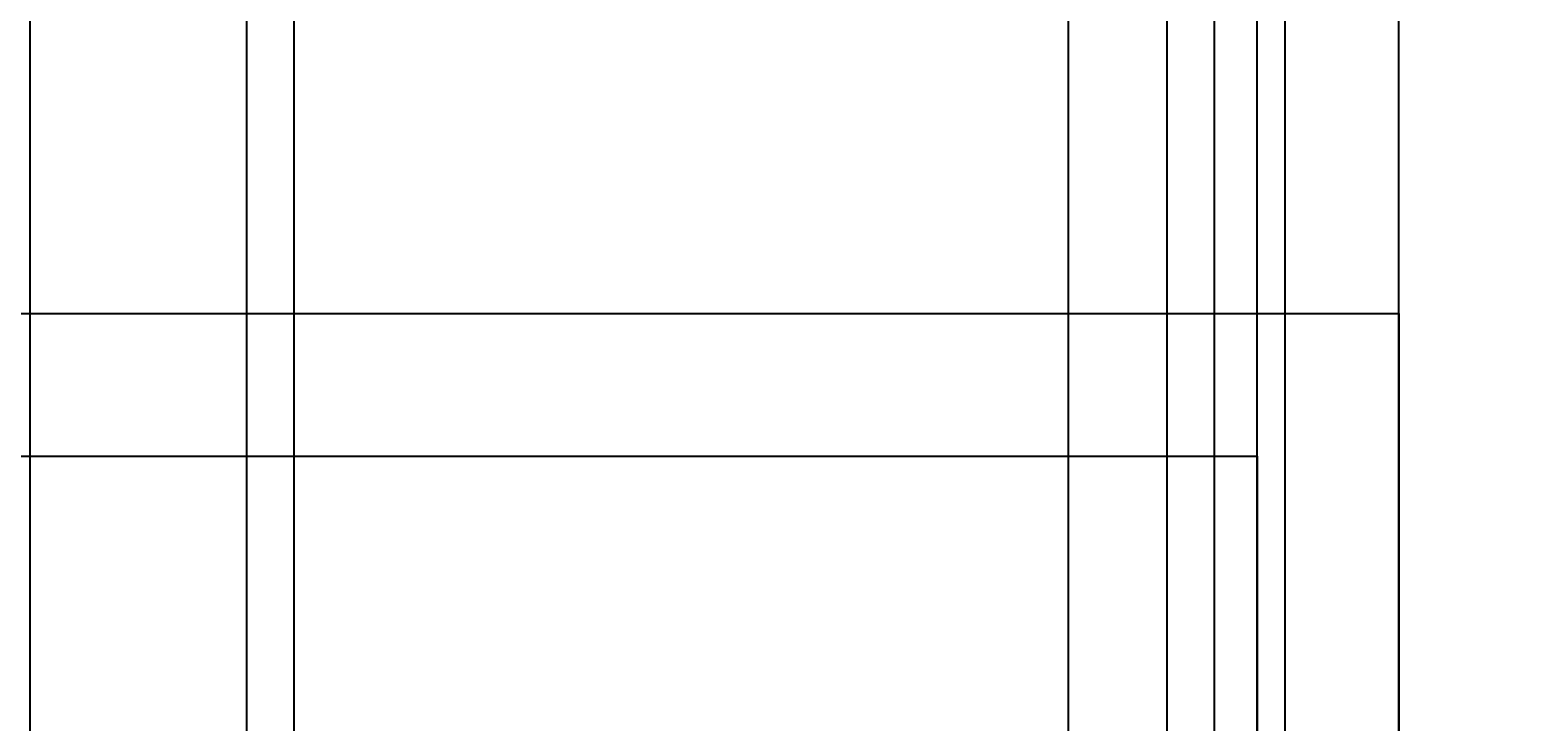
# Model space of a CAD drawing. Units: inches. Extents: x -6 to 289, y -8 to 323.
# Tile 27 of 107: x 142 to 174, y 109 to 124. Entities that reach past the tile are written whole.
import ezdxf

# ---------------------------------------------------------------- set-up
doc = ezdxf.new("R2010")
doc.units = ezdxf.units.IN
doc.header["$MEASUREMENT"] = 0
doc.layers.add('A-ANNO-DIMS', color=2, linetype='Continuous', lineweight=18)
doc.layers.add('A-DOOR', color=3, linetype='Continuous', lineweight=25)
doc.styles.get("Standard").update_dxf_attribs({"font": 'arial.ttf'})
doc.dimstyles.get("Standard").update_dxf_attribs({"dimtxt": 0.18, "dimasz": 0.18, "dimexe": 0.18, "dimexo": 0.0625, "dimgap": 0.09, "dimtad": 0, "dimtih": 1, "dimtoh": 1, "dimdec": 4, "dimzin": 0, "dimdsep": 46, "dimtxsty": 'Standard', "dimcen": 0.09, "dimadec": 0, "dimazin": 0, "dimtfac": 1, "dimtdec": 4, "dimtofl": 0, "dimtmove": 0, "dimatfit": 3, "dimfxl": 1, "dimtolj": 1, "dimtzin": 0, "dimarcsym": 0})

# ---------------------------------------------------------------- blocks, each defined once
blk = doc.blocks.new('*D30')
at = {"layer": 'A-ANNO-DIMS', "color": 0, "lineweight": -2, "transparency": 16777216}
for p, q in [((129.383, 181.092), (129.383, -8.391)), ((146.883, 181.092), (146.883, -8.391)), ((129.563, -8.211), (137.817, -8.211)), ((146.703, -8.211), (138.449, -8.211))]:
    blk.add_line(p, q, dxfattribs=at)
at = {"layer": 'A-ANNO-DIMS', "color": 0, "transparency": 16777216}
for points in [[(129.563, -8.181), (129.563, -8.241), (129.383, -8.211)], [(146.703, -8.181), (146.703, -8.241), (146.883, -8.211)]]:
    blk.add_solid(points, dxfattribs=at)
at = {"layer": 'Defpoints', "color": 0, "transparency": 16777216}
for p in [(129.383, 181.154), (146.883, 181.154), (146.883, -8.211)]:
    blk.add_point(p, dxfattribs=at)
at = {"layer": 'A-ANNO-DIMS', "color": 0, "transparency": 16777216, "insert": (138.133, -8.211), "char_height": 0.18, "attachment_point": 5}
blk.add_mtext('\\A1;17.5', dxfattribs=at)
blk = doc.blocks.new('*D31')
at = {"layer": 'A-ANNO-DIMS', "color": 0, "lineweight": -2, "transparency": 16777216}
for p, q in [((146.883, 181.092), (146.883, -8.391)), ((147.883, 181.092), (147.883, -8.391)), ((147.063, -8.211), (147.26, -8.211)), ((147.703, -8.211), (147.507, -8.211))]:
    blk.add_line(p, q, dxfattribs=at)
at = {"layer": 'A-ANNO-DIMS', "color": 0, "transparency": 16777216}
for points in [[(147.063, -8.181), (147.063, -8.241), (146.883, -8.211)], [(147.703, -8.181), (147.703, -8.241), (147.883, -8.211)]]:
    blk.add_solid(points, dxfattribs=at)
at = {"layer": 'Defpoints', "color": 0, "transparency": 16777216}
for p in [(146.883, 181.154), (147.883, 181.154), (147.883, -8.211)]:
    blk.add_point(p, dxfattribs=at)
at = {"layer": 'A-ANNO-DIMS', "color": 0, "transparency": 16777216, "insert": (147.383, -8.211), "char_height": 0.18, "attachment_point": 5}
blk.add_mtext('\\A1;1', dxfattribs=at)
blk = doc.blocks.new('*D32')
at = {"layer": 'A-ANNO-DIMS', "color": 0, "lineweight": -2, "transparency": 16777216}
for p, q in [((147.883, 181.092), (147.883, -8.391)), ((166.383, 181.092), (166.383, -8.391)), ((148.063, -8.211), (156.817, -8.211)), ((166.203, -8.211), (157.449, -8.211))]:
    blk.add_line(p, q, dxfattribs=at)
at = {"layer": 'A-ANNO-DIMS', "color": 0, "transparency": 16777216}
for points in [[(148.063, -8.181), (148.063, -8.241), (147.883, -8.211)], [(166.203, -8.181), (166.203, -8.241), (166.383, -8.211)]]:
    blk.add_solid(points, dxfattribs=at)
at = {"layer": 'Defpoints', "color": 0, "transparency": 16777216}
for p in [(147.883, 181.154), (166.383, 181.154), (166.383, -8.211)]:
    blk.add_point(p, dxfattribs=at)
at = {"layer": 'A-ANNO-DIMS', "color": 0, "transparency": 16777216, "insert": (157.133, -8.211), "char_height": 0.18, "attachment_point": 5}
blk.add_mtext('\\A1;18.5', dxfattribs=at)
blk = doc.blocks.new('*D33')
at = {"layer": 'A-ANNO-DIMS', "color": 0, "lineweight": -2, "transparency": 16777216}
for p, q in [((166.383, 181.092), (166.383, -8.391)), ((167.383, 180.092), (167.383, -8.391)), ((166.563, -8.211), (166.76, -8.211)), ((167.203, -8.211), (167.007, -8.211))]:
    blk.add_line(p, q, dxfattribs=at)
at = {"layer": 'A-ANNO-DIMS', "color": 0, "transparency": 16777216}
for points in [[(166.563, -8.181), (166.563, -8.241), (166.383, -8.211)], [(167.203, -8.181), (167.203, -8.241), (167.383, -8.211)]]:
    blk.add_solid(points, dxfattribs=at)
at = {"layer": 'Defpoints', "color": 0, "transparency": 16777216}
for p in [(166.383, 181.154), (167.383, 180.154), (167.383, -8.211)]:
    blk.add_point(p, dxfattribs=at)
at = {"layer": 'A-ANNO-DIMS', "color": 0, "transparency": 16777216, "insert": (166.883, -8.211), "char_height": 0.18, "attachment_point": 5}
blk.add_mtext('\\A1;1', dxfattribs=at)
blk = doc.blocks.new('*D34')
at = {"layer": 'A-ANNO-DIMS', "color": 0, "lineweight": -2, "transparency": 16777216}
for p, q in [((167.383, 180.092), (167.383, -8.391)), ((168.883, 178.592), (168.883, -8.391)), ((167.563, -8.211), (167.887, -8.211)), ((168.703, -8.211), (168.38, -8.211))]:
    blk.add_line(p, q, dxfattribs=at)
at = {"layer": 'A-ANNO-DIMS', "color": 0, "transparency": 16777216}
for points in [[(167.563, -8.181), (167.563, -8.241), (167.383, -8.211)], [(168.703, -8.181), (168.703, -8.241), (168.883, -8.211)]]:
    blk.add_solid(points, dxfattribs=at)
at = {"layer": 'Defpoints', "color": 0, "transparency": 16777216}
for p in [(167.383, 180.154), (168.883, 178.654), (168.883, -8.211)]:
    blk.add_point(p, dxfattribs=at)
at = {"layer": 'A-ANNO-DIMS', "color": 0, "transparency": 16777216, "insert": (168.133, -8.211), "char_height": 0.18, "attachment_point": 5}
blk.add_mtext('\\A1;1.5', dxfattribs=at)
blk = doc.blocks.new('*D76')
at = {"layer": 'A-ANNO-DIMS', "color": 0, "lineweight": -2, "transparency": 16777216}
for p, q in [((142.296, 51.148), (142.296, 322.969)), ((142.476, 322.789), (153.076, 322.789)), ((164.116, 322.789), (153.516, 322.789)), ((164.296, 51.148), (164.296, 322.969))]:
    blk.add_line(p, q, dxfattribs=at)
at = {"layer": 'A-ANNO-DIMS', "color": 0, "transparency": 16777216}
for points in [[(142.476, 322.819), (142.476, 322.759), (142.296, 322.789)], [(164.116, 322.819), (164.116, 322.759), (164.296, 322.789)]]:
    blk.add_solid(points, dxfattribs=at)
at = {"layer": 'Defpoints', "color": 0, "transparency": 16777216}
for p in [(164.296, 322.789), (142.296, 51.085), (164.296, 51.085)]:
    blk.add_point(p, dxfattribs=at)
at = {"layer": 'A-ANNO-DIMS', "color": 0, "transparency": 16777216, "insert": (153.296, 322.789), "char_height": 0.18, "attachment_point": 5}
blk.add_mtext('\\A1;22', dxfattribs=at)
blk = doc.blocks.new('*D77')
at = {"layer": 'A-ANNO-DIMS', "color": 0, "lineweight": -2, "transparency": 16777216}
for p, q in [((164.296, 51.148), (164.296, 322.969)), ((164.476, 322.789), (166.144, 322.789)), ((168.116, 322.789), (166.448, 322.789)), ((168.296, 51.148), (168.296, 322.969))]:
    blk.add_line(p, q, dxfattribs=at)
at = {"layer": 'A-ANNO-DIMS', "color": 0, "transparency": 16777216}
for points in [[(164.476, 322.819), (164.476, 322.759), (164.296, 322.789)], [(168.116, 322.819), (168.116, 322.759), (168.296, 322.789)]]:
    blk.add_solid(points, dxfattribs=at)
at = {"layer": 'Defpoints', "color": 0, "transparency": 16777216}
for p in [(168.296, 322.789), (164.296, 51.085), (168.296, 51.085)]:
    blk.add_point(p, dxfattribs=at)
at = {"layer": 'A-ANNO-DIMS', "color": 0, "transparency": 16777216, "insert": (166.296, 322.789), "char_height": 0.18, "attachment_point": 5}
blk.add_mtext('\\A1;4', dxfattribs=at)
blk = doc.blocks.new('*D78')
at = {"layer": 'A-ANNO-DIMS', "color": 0, "lineweight": -2, "transparency": 16777216}
for p, q in [((168.296, 51.148), (168.296, 322.969)), ((168.476, 322.789), (169.647, 322.789)), ((171.116, 322.789), (169.945, 322.789)), ((171.296, 51.148), (171.296, 322.969))]:
    blk.add_line(p, q, dxfattribs=at)
at = {"layer": 'A-ANNO-DIMS', "color": 0, "transparency": 16777216}
for points in [[(168.476, 322.819), (168.476, 322.759), (168.296, 322.789)], [(171.116, 322.819), (171.116, 322.759), (171.296, 322.789)]]:
    blk.add_solid(points, dxfattribs=at)
at = {"layer": 'Defpoints', "color": 0, "transparency": 16777216}
for p in [(171.296, 322.789), (168.296, 51.085), (171.296, 51.085)]:
    blk.add_point(p, dxfattribs=at)
at = {"layer": 'A-ANNO-DIMS', "color": 0, "transparency": 16777216, "insert": (169.796, 322.789), "char_height": 0.18, "attachment_point": 5}
blk.add_mtext('\\A1;3', dxfattribs=at)
blk = doc.blocks.new('*D79')
at = {"layer": 'A-ANNO-DIMS', "color": 0, "lineweight": -2, "transparency": 16777216}
for p, q in [((171.296, 118.033), (171.296, 322.969)), ((171.476, 322.789), (179.339, 322.789)), ((188.112, 322.789), (180.249, 322.789)), ((188.292, 116.842), (188.292, 322.969))]:
    blk.add_line(p, q, dxfattribs=at)
at = {"layer": 'A-ANNO-DIMS', "color": 0, "transparency": 16777216}
for points in [[(171.476, 322.819), (171.476, 322.759), (171.296, 322.789)], [(188.112, 322.819), (188.112, 322.759), (188.292, 322.789)]]:
    blk.add_solid(points, dxfattribs=at)
at = {"layer": 'Defpoints', "color": 0, "transparency": 16777216}
for p in [(188.292, 322.789), (171.296, 117.971), (188.292, 116.779)]:
    blk.add_point(p, dxfattribs=at)
at = {"layer": 'A-ANNO-DIMS', "color": 0, "transparency": 16777216, "insert": (179.794, 322.789), "char_height": 0.18, "attachment_point": 5}
blk.add_mtext('\\A1;16.996', dxfattribs=at)

msp = doc.modelspace()

# ---------------------------------------------------------------- linework, layer by layer
at = {"layer": 'A-DOOR'}
for points in [[(135.296, 51.0851), (135.296, 117.9706), (171.296, 117.9706), (171.296, 51.0851)], [(138.296, 51.0851), (138.296, 114.9477), (168.296, 114.9477), (168.296, 51.0851)]]:
    msp.add_lwpolyline(points, dxfattribs=at)

# ---------------------------------------------------------------- dimensions: what is measured, and where the dimension line sits
at = {"layer": 'A-ANNO-DIMS'}
for base, p1, p2, override, picture, middle in [((164.296, 322.7888), (142.296, 51.0851), (164.296, 51.0851), {"dimdec": 0, "dimlfac": 1, "dimrnd": 0, "dimzin": 0, "dimdsep": 46, "dimlunit": 2}, '*D76', (153.296, 322.7888)), ((168.296, 322.7888), (164.296, 51.0851), (168.296, 51.0851), {"dimdec": 0, "dimlfac": 1, "dimrnd": 0, "dimzin": 0, "dimdsep": 46, "dimlunit": 2}, '*D77', (166.296, 322.7888)), ((171.296, 322.7888), (168.296, 51.0851), (171.296, 51.0851), {"dimdec": 0, "dimlfac": 1, "dimrnd": 0, "dimzin": 0, "dimdsep": 46, "dimlunit": 2}, '*D78', (169.796, 322.7888)), ((188.2918, 322.7888), (171.296, 117.9706), (188.2918, 116.7795), {"dimdec": 3, "dimlfac": 1, "dimrnd": 0, "dimzin": 0, "dimdsep": 46, "dimlunit": 2}, '*D79', (179.7939, 322.7888)), ((146.8835, -8.2112), (129.3835, 181.154), (146.8835, 181.154), {"dimdec": 1, "dimlfac": 1, "dimrnd": 0, "dimzin": 0, "dimdsep": 46, "dimlunit": 2}, '*D30', (138.1335, -8.2112)), ((147.8835, -8.2112), (146.8835, 181.154), (147.8835, 181.154), {"dimdec": 0, "dimlfac": 1, "dimrnd": 0, "dimzin": 0, "dimdsep": 46, "dimlunit": 2}, '*D31', (147.3835, -8.2112)), ((166.3835, -8.2112), (147.8835, 181.154), (166.3835, 181.154), {"dimdec": 1, "dimlfac": 1, "dimrnd": 0, "dimzin": 0, "dimdsep": 46, "dimlunit": 2}, '*D32', (157.1335, -8.2112)), ((167.3835, -8.2112), (166.3835, 181.154), (167.3835, 180.154), {"dimdec": 0, "dimlfac": 1, "dimrnd": 0, "dimzin": 0, "dimdsep": 46, "dimlunit": 2}, '*D33', (166.8835, -8.2112)), ((168.8835, -8.2112), (167.3835, 180.154), (168.8835, 178.654), {"dimdec": 1, "dimlfac": 1, "dimrnd": 0, "dimzin": 0, "dimdsep": 46, "dimlunit": 2}, '*D34', (168.1335, -8.2112))]:
    dim = msp.add_linear_dim(base=base, p1=p1, p2=p2, dimstyle='Standard', override=override, dxfattribs=at)
    dim.commit()
    dim.dimension.update_dxf_attribs({"geometry": picture, "text_midpoint": middle})

doc.saveas('drawing.dxf')
